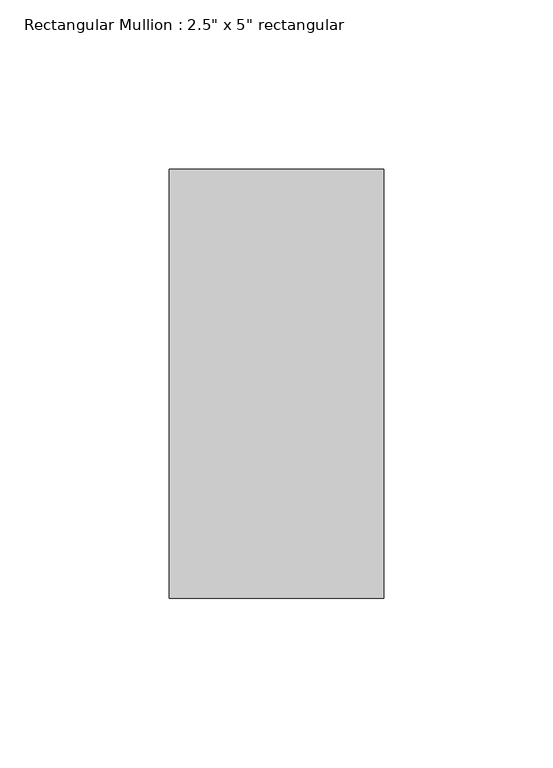
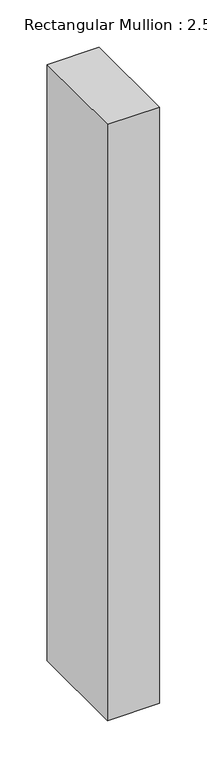
"""IFC4 building model written with IfcOpenShell, lengths in millimetres: member geometry."""

from ifc_helpers import new_model, si_unit, frame, origin, place, context, project, spatial, polyline, outline, extrude, source, transform, mapped, element, save


def member_29a45e76(model_context):
    return source(origin(), model_context, "Body", "SweptSolid", [
        extrude(outline(polyline([(0.0, 63.5), (0.0, -63.5), (-63.5, -63.5), (-63.5, 63.5), (0.0, 63.5)])), frame((0.0, 0.0, -768.0046847), z_axis=(0.0, 0.0, 1.0), x_axis=(1.0, 0.0, 0.0)), (0.0, 0.0, 1.0), 768.0046847),
    ])


if __name__ == "__main__":
    model = new_model("IFC4")
    model_context = context("Model", 3, world=origin())
    ifc_project = project(units=[si_unit("LENGTHUNIT", "METRE", prefix="MILLI")], contexts=[model_context])
    site = spatial("IfcSite", under=ifc_project)
    building = spatial("IfcBuilding", under=site)
    placement = place(None, origin())
    member_shape = member_29a45e76(model_context)
    element("IfcMember", 1, ObjectType="Rectangular Mullion : 2.5\" x 5\" rectangular", at=placement, inside=building, context=model_context, shape_type="MappedRepresentation", body=[
        mapped(member_shape, transform((0.0, 0.0, 0.0), x_axis=(1.0, 0.0, 0.0), y_axis=(0.0, 1.0, 0.0), z_axis=(0.0, 0.0, 1.0))),
    ])
    save(model, "model.ifc")

# Revit data of these elements
# Type "Rectangular Mullion : 2.5\" x 5\" rectangular"
#   built-in parameter 1007304 = 0.416667 (stored number, unit not read)
#   built-in parameter 1007301 = 0.104167 (stored number, unit not read)
#   built-in parameter 1007300 = 0.104167 (stored number, unit not read)
# Element 1 (IfcMember, "Rectangular Mullion : 2.5\" x 5\" rectangular")
#   Materials on its faces: "Aluminum"
# Materials
#   "Aluminum": class "Metal", colour RGB 247 247 247, transparency 0, Description = "Aluminum 6061", Cost = 0
